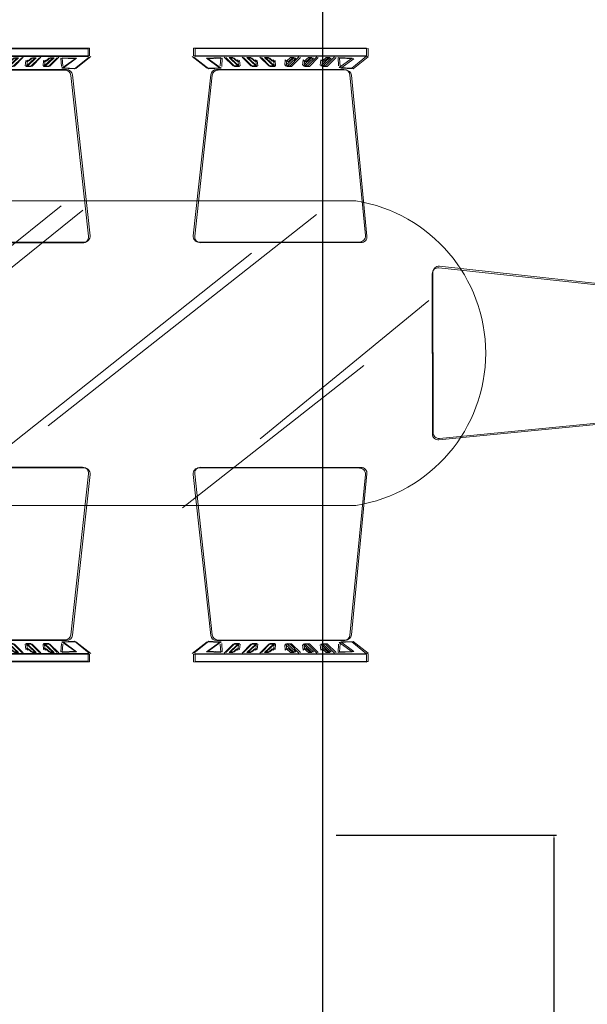
# Model space of a CAD drawing. Units: inches. Extents: x -26 to 575, y -18 to 513.
# Tile 20 of 28: x 316 to 355, y 241 to 307. Entities that reach past the tile are written whole.
import ezdxf

# ---------------------------------------------------------------- set-up
doc = ezdxf.new("R2010")
doc.units = ezdxf.units.IN
doc.header["$MEASUREMENT"] = 0
doc.layers.add('A-ANNO-DIMS', color=2, linetype='Continuous', lineweight=18)
doc.layers.add('Furniture', color=8, linetype='Continuous', lineweight=15)
doc.styles.get("Standard").update_dxf_attribs({"font": 'arial.ttf', "height": 6})
doc.dimstyles.get("Standard").update_dxf_attribs({"dimtxt": 6, "dimasz": 0.18, "dimexe": 0.18, "dimexo": 0.0625, "dimgap": 0.09, "dimtad": 0, "dimtih": 1, "dimtoh": 1, "dimzin": 0, "dimdsep": 46, "dimlunit": 3, "dimtxsty": 'Standard', "dimcen": 0.09, "dimadec": 0, "dimazin": 0, "dimtfac": 1, "dimtofl": 0, "dimtmove": 0, "dimatfit": 3, "dimfxl": 1, "dimtolj": 1, "dimtzin": 0, "dimarcsym": 0})

# ---------------------------------------------------------------- blocks, each defined once
blk = doc.blocks.new('DINING-SET-6-SEAT')
for p, q in [((16.828, 40.76, -3.573), (16.828, 41.278, -3.573)), ((16.828, 41.278, -3.573), (28.461, 41.278, -3.573)), ((16.931, 40.798, -3.573), (16.931, 41.316, -3.573)), ((16.931, 41.316, -3.573), (28.564, 41.316, -3.573)), ((28.461, 41.278, -3.573), (28.461, 40.76, -3.573)), ((28.564, 41.316, -3.573), (28.564, 40.798, -3.573)), ((47.187, 41.329, -3.573), (35.554, 41.319, -3.573)), ((35.554, 41.319, -3.573), (35.554, 40.801, -3.573)), ((47.29, 41.291, -3.573), (35.657, 41.281, -3.573)), ((35.657, 41.281, -3.573), (35.657, 40.763, -3.573)), ((47.188, 40.811, -3.573), (47.187, 41.329, -3.573)), ((47.29, 40.774, -3.573), (47.29, 41.291, -3.573)), ((28.461, 40.76, -3.573), (16.828, 40.76, -3.573)), ((16.828, 40.72, -3.573), (17.824, 39.924, -3.573)), ((28.564, 40.798, -3.573), (16.931, 40.798, -3.573)), ((16.931, 40.758, -3.573), (17.927, 39.962, -3.573)), ((17.784, 40.601, -3.573), (18.74, 40.641, -3.573)), ((18.661, 39.964, -3.573), (17.784, 40.601, -3.573)), ((17.887, 40.639, -3.573), (18.843, 40.679, -3.573)), ((18.763, 40.002, -3.573), (17.887, 40.639, -3.573)), ((18.74, 40.641, -3.573), (18.7, 40.083, -3.573)), ((18.843, 40.679, -3.573), (18.803, 40.121, -3.573)), ((18.979, 40.681, -3.573), (19.577, 40.083, -3.573)), ((19.082, 40.718, -3.573), (19.68, 40.121, -3.573)), ((19.896, 40.083, -3.573), (19.298, 40.641, -3.573)), ((19.298, 40.641, -3.573), (19.537, 40.641, -3.573)), ((19.998, 40.121, -3.573), (19.401, 40.679, -3.573)), ((19.401, 40.679, -3.573), (19.64, 40.679, -3.573)), ((19.537, 40.641, -3.573), (19.816, 40.402, -3.573)), ((19.64, 40.679, -3.573), (19.919, 40.44, -3.573)), ((19.816, 40.402, -3.573), (19.896, 40.481, -3.573)), ((19.896, 40.481, -3.573), (19.936, 40.123, -3.573)), ((19.919, 40.44, -3.573), (19.998, 40.519, -3.573)), ((19.998, 40.519, -3.573), (20.038, 40.161, -3.573)), ((20.175, 40.681, -3.573), (20.772, 40.083, -3.573)), ((20.277, 40.718, -3.573), (20.875, 40.121, -3.573)), ((21.091, 40.083, -3.573), (20.493, 40.641, -3.573)), ((20.493, 40.641, -3.573), (20.732, 40.641, -3.573)), ((21.194, 40.121, -3.573), (20.596, 40.679, -3.573)), ((20.596, 40.679, -3.573), (20.835, 40.679, -3.573)), ((20.732, 40.641, -3.573), (21.011, 40.402, -3.573)), ((20.835, 40.679, -3.573), (21.114, 40.44, -3.573)), ((21.011, 40.402, -3.573), (21.091, 40.481, -3.573)), ((21.091, 40.481, -3.573), (21.131, 40.123, -3.573)), ((21.114, 40.44, -3.573), (21.194, 40.519, -3.573)), ((21.194, 40.519, -3.573), (21.233, 40.161, -3.573)), ((21.37, 40.681, -3.573), (21.967, 40.083, -3.573)), ((21.473, 40.718, -3.573), (22.07, 40.121, -3.573)), ((22.286, 40.083, -3.573), (21.688, 40.641, -3.573)), ((21.688, 40.641, -3.573), (21.928, 40.641, -3.573)), ((22.389, 40.121, -3.573), (21.791, 40.679, -3.573)), ((21.791, 40.679, -3.573), (22.03, 40.679, -3.573)), ((21.928, 40.641, -3.573), (22.206, 40.402, -3.573)), ((22.03, 40.679, -3.573), (22.309, 40.44, -3.573)), ((22.206, 40.402, -3.573), (22.286, 40.481, -3.573)), ((22.286, 40.481, -3.573), (22.326, 40.123, -3.573)), ((22.309, 40.44, -3.573), (22.389, 40.519, -3.573)), ((22.389, 40.519, -3.573), (22.429, 40.161, -3.573)), ((23.083, 40.481, -3.573), (23.043, 40.123, -3.573)), ((23.083, 40.083, -3.573), (23.681, 40.641, -3.573)), ((23.163, 40.402, -3.573), (23.083, 40.481, -3.573)), ((23.186, 40.519, -3.573), (23.146, 40.161, -3.573)), ((23.441, 40.641, -3.573), (23.163, 40.402, -3.573)), ((23.186, 40.121, -3.573), (23.783, 40.679, -3.573)), ((23.265, 40.44, -3.573), (23.186, 40.519, -3.573)), ((23.544, 40.679, -3.573), (23.265, 40.44, -3.573)), ((23.999, 40.681, -3.573), (23.402, 40.083, -3.573)), ((23.681, 40.641, -3.573), (23.441, 40.641, -3.573)), ((24.102, 40.718, -3.573), (23.504, 40.121, -3.573)), ((23.783, 40.679, -3.573), (23.544, 40.679, -3.573)), ((24.278, 40.481, -3.573), (24.238, 40.123, -3.573)), ((24.278, 40.083, -3.573), (24.876, 40.641, -3.573)), ((24.358, 40.402, -3.573), (24.278, 40.481, -3.573)), ((24.381, 40.519, -3.573), (24.341, 40.161, -3.573)), ((24.637, 40.641, -3.573), (24.358, 40.402, -3.573)), ((24.381, 40.121, -3.573), (24.978, 40.679, -3.573)), ((24.461, 40.44, -3.573), (24.381, 40.519, -3.573)), ((24.739, 40.679, -3.573), (24.461, 40.44, -3.573)), ((25.194, 40.681, -3.573), (24.597, 40.083, -3.573)), ((24.876, 40.641, -3.573), (24.637, 40.641, -3.573)), ((25.297, 40.718, -3.573), (24.7, 40.121, -3.573)), ((24.978, 40.679, -3.573), (24.739, 40.679, -3.573)), ((25.473, 40.481, -3.573), (25.434, 40.123, -3.573)), ((25.473, 40.083, -3.573), (26.071, 40.641, -3.573)), ((25.553, 40.402, -3.573), (25.473, 40.481, -3.573)), ((25.576, 40.519, -3.573), (25.536, 40.161, -3.573)), ((25.832, 40.641, -3.573), (25.553, 40.402, -3.573)), ((25.576, 40.121, -3.573), (26.174, 40.679, -3.573)), ((25.656, 40.44, -3.573), (25.576, 40.519, -3.573)), ((25.935, 40.679, -3.573), (25.656, 40.44, -3.573)), ((26.39, 40.681, -3.573), (25.792, 40.083, -3.573)), ((26.071, 40.641, -3.573), (25.832, 40.641, -3.573)), ((26.492, 40.718, -3.573), (25.895, 40.121, -3.573)), ((26.174, 40.679, -3.573), (25.935, 40.679, -3.573)), ((27.585, 40.601, -3.573), (26.629, 40.641, -3.573)), ((26.629, 40.641, -3.573), (26.669, 40.083, -3.573)), ((26.708, 39.964, -3.573), (27.585, 40.601, -3.573)), ((27.688, 40.639, -3.573), (26.731, 40.679, -3.573)), ((26.731, 40.679, -3.573), (26.771, 40.121, -3.573)), ((26.811, 40.002, -3.573), (27.688, 40.639, -3.573)), ((28.541, 40.72, -3.573), (27.545, 39.924, -3.573)), ((28.644, 40.758, -3.573), (27.648, 39.962, -3.573)), ((35.475, 40.761, -3.573), (36.471, 39.966, -3.573)), ((35.554, 40.801, -3.573), (47.188, 40.811, -3.573)), ((35.577, 40.723, -3.573), (36.574, 39.928, -3.573)), ((35.657, 40.763, -3.573), (47.29, 40.774, -3.573)), ((36.431, 40.643, -3.573), (37.387, 40.683, -3.573)), ((37.308, 40.006, -3.573), (36.431, 40.643, -3.573)), ((36.534, 40.605, -3.573), (37.49, 40.646, -3.573)), ((37.411, 39.968, -3.573), (36.534, 40.605, -3.573)), ((37.387, 40.683, -3.573), (37.348, 40.126, -3.573)), ((37.49, 40.646, -3.573), (37.45, 40.088, -3.573)), ((37.626, 40.723, -3.573), (38.224, 40.127, -3.573)), ((37.729, 40.686, -3.573), (38.327, 40.089, -3.573)), ((38.543, 40.127, -3.573), (37.945, 40.684, -3.573)), ((37.945, 40.684, -3.573), (38.184, 40.684, -3.573)), ((38.646, 40.089, -3.573), (38.048, 40.646, -3.573)), ((38.048, 40.646, -3.573), (38.287, 40.646, -3.573)), ((38.184, 40.684, -3.573), (38.463, 40.445, -3.573)), ((38.287, 40.646, -3.573), (38.566, 40.408, -3.573)), ((38.463, 40.445, -3.573), (38.543, 40.525, -3.573)), ((38.543, 40.525, -3.573), (38.583, 40.167, -3.573)), ((38.566, 40.408, -3.573), (38.645, 40.487, -3.573)), ((38.645, 40.487, -3.573), (38.685, 40.129, -3.573)), ((38.821, 40.724, -3.573), (39.419, 40.128, -3.573)), ((38.924, 40.687, -3.573), (39.522, 40.09, -3.573)), ((39.738, 40.128, -3.573), (39.14, 40.685, -3.573)), ((39.14, 40.685, -3.573), (39.379, 40.685, -3.573)), ((39.841, 40.09, -3.573), (39.243, 40.647, -3.573)), ((39.243, 40.647, -3.573), (39.482, 40.647, -3.573)), ((39.379, 40.685, -3.573), (39.658, 40.446, -3.573)), ((39.482, 40.647, -3.573), (39.761, 40.409, -3.573)), ((39.658, 40.446, -3.573), (39.738, 40.526, -3.573)), ((39.738, 40.526, -3.573), (39.778, 40.168, -3.573)), ((39.761, 40.409, -3.573), (39.841, 40.488, -3.573)), ((39.841, 40.488, -3.573), (39.881, 40.13, -3.573)), ((40.016, 40.725, -3.573), (40.615, 40.129, -3.573)), ((40.119, 40.688, -3.573), (40.717, 40.091, -3.573)), ((40.933, 40.129, -3.573), (40.335, 40.686, -3.573)), ((40.335, 40.686, -3.573), (40.574, 40.686, -3.573)), ((41.036, 40.091, -3.573), (40.438, 40.648, -3.573)), ((40.438, 40.648, -3.573), (40.677, 40.648, -3.573)), ((40.574, 40.686, -3.573), (40.853, 40.447, -3.573)), ((40.677, 40.648, -3.573), (40.956, 40.41, -3.573)), ((40.853, 40.447, -3.573), (40.933, 40.527, -3.573)), ((40.933, 40.527, -3.573), (40.973, 40.169, -3.573)), ((40.956, 40.41, -3.573), (41.036, 40.489, -3.573)), ((41.036, 40.489, -3.573), (41.076, 40.131, -3.573)), ((41.73, 40.528, -3.573), (41.69, 40.169, -3.573)), ((41.73, 40.13, -3.573), (42.327, 40.688, -3.573)), ((41.81, 40.448, -3.573), (41.73, 40.528, -3.573)), ((41.833, 40.49, -3.573), (41.793, 40.132, -3.573)), ((42.088, 40.687, -3.573), (41.81, 40.448, -3.573)), ((41.833, 40.092, -3.573), (42.43, 40.65, -3.573)), ((41.912, 40.41, -3.573), (41.833, 40.49, -3.573)), ((42.191, 40.65, -3.573), (41.912, 40.41, -3.573)), ((42.646, 40.728, -3.573), (42.049, 40.13, -3.573)), ((42.327, 40.688, -3.573), (42.088, 40.687, -3.573)), ((42.749, 40.69, -3.573), (42.152, 40.092, -3.573)), ((42.43, 40.65, -3.573), (42.191, 40.65, -3.573)), ((42.925, 40.529, -3.573), (42.885, 40.17, -3.573)), ((42.925, 40.131, -3.573), (43.522, 40.689, -3.573)), ((43.005, 40.449, -3.573), (42.925, 40.529, -3.573)), ((43.028, 40.491, -3.573), (42.988, 40.133, -3.573)), ((43.283, 40.688, -3.573), (43.005, 40.449, -3.573)), ((43.028, 40.093, -3.573), (43.625, 40.651, -3.573)), ((43.108, 40.412, -3.573), (43.028, 40.491, -3.573)), ((43.386, 40.651, -3.573), (43.108, 40.412, -3.573)), ((43.841, 40.729, -3.573), (43.244, 40.131, -3.573)), ((43.522, 40.689, -3.573), (43.283, 40.688, -3.573)), ((43.944, 40.691, -3.573), (43.347, 40.093, -3.573)), ((43.625, 40.651, -3.573), (43.386, 40.651, -3.573)), ((44.12, 40.53, -3.573), (44.081, 40.171, -3.573)), ((44.2, 40.45, -3.573), (44.12, 40.53, -3.573)), ((44.121, 40.132, -3.573), (44.718, 40.69, -3.573)), ((44.223, 40.492, -3.573), (44.183, 40.134, -3.573)), ((44.479, 40.69, -3.573), (44.2, 40.45, -3.573)), ((44.223, 40.094, -3.573), (44.82, 40.652, -3.573)), ((44.303, 40.413, -3.573), (44.223, 40.492, -3.573)), ((44.581, 40.652, -3.573), (44.303, 40.413, -3.573)), ((45.036, 40.73, -3.573), (44.439, 40.132, -3.573)), ((44.718, 40.69, -3.573), (44.479, 40.69, -3.573)), ((45.139, 40.692, -3.573), (44.542, 40.094, -3.573)), ((44.82, 40.652, -3.573), (44.581, 40.652, -3.573)), ((46.232, 40.651, -3.573), (45.275, 40.69, -3.573)), ((45.275, 40.69, -3.573), (45.316, 40.133, -3.573)), ((45.356, 40.013, -3.573), (46.232, 40.651, -3.573)), ((46.334, 40.613, -3.573), (45.378, 40.652, -3.573)), ((45.378, 40.652, -3.573), (45.419, 40.095, -3.573)), ((45.458, 39.976, -3.573), (46.334, 40.613, -3.573)), ((47.188, 40.772, -3.573), (46.192, 39.974, -3.573)), ((47.29, 40.734, -3.573), (46.295, 39.936, -3.573)), ((17.824, 39.924, -3.573), (18.661, 39.964, -3.573)), ((17.927, 39.962, -3.573), (18.763, 40.002, -3.573)), ((26.909, 39.844, -3.573), (18.345, 39.844, -3.573)), ((27.012, 39.882, -3.573), (18.448, 39.882, -3.573)), ((19.577, 40.083, -3.573), (19.896, 40.083, -3.573)), ((19.68, 40.121, -3.573), (19.998, 40.121, -3.573)), ((20.772, 40.083, -3.573), (21.091, 40.083, -3.573)), ((20.875, 40.121, -3.573), (21.194, 40.121, -3.573)), ((21.967, 40.083, -3.573), (22.286, 40.083, -3.573)), ((22.07, 40.121, -3.573), (22.389, 40.121, -3.573)), ((23.402, 40.083, -3.573), (23.083, 40.083, -3.573)), ((23.504, 40.121, -3.573), (23.186, 40.121, -3.573)), ((24.597, 40.083, -3.573), (24.278, 40.083, -3.573)), ((24.7, 40.121, -3.573), (24.381, 40.121, -3.573)), ((25.792, 40.083, -3.573), (25.473, 40.083, -3.573)), ((25.895, 40.121, -3.573), (25.576, 40.121, -3.573)), ((27.545, 39.924, -3.573), (26.708, 39.964, -3.573)), ((27.648, 39.962, -3.573), (26.811, 40.002, -3.573)), ((36.471, 39.966, -3.573), (37.308, 40.006, -3.573)), ((36.574, 39.928, -3.573), (37.411, 39.968, -3.573)), ((37.107, 39.887, -3.573), (45.671, 39.894, -3.573)), ((37.21, 39.849, -3.573), (45.774, 39.856, -3.573)), ((38.224, 40.127, -3.573), (38.543, 40.127, -3.573)), ((38.327, 40.089, -3.573), (38.646, 40.089, -3.573)), ((39.419, 40.128, -3.573), (39.738, 40.128, -3.573)), ((39.522, 40.09, -3.573), (39.841, 40.09, -3.573)), ((40.615, 40.129, -3.573), (40.933, 40.129, -3.573)), ((40.717, 40.091, -3.573), (41.036, 40.091, -3.573)), ((42.049, 40.13, -3.573), (41.73, 40.13, -3.573)), ((42.152, 40.092, -3.573), (41.833, 40.092, -3.573)), ((43.244, 40.131, -3.573), (42.925, 40.131, -3.573)), ((43.347, 40.093, -3.573), (43.028, 40.093, -3.573)), ((44.439, 40.132, -3.573), (44.121, 40.132, -3.573)), ((44.542, 40.094, -3.573), (44.223, 40.094, -3.573)), ((46.192, 39.974, -3.573), (45.356, 40.013, -3.573)), ((46.295, 39.936, -3.573), (45.458, 39.976, -3.573)), ((17.949, 39.484, -3.573), (16.91, 28.653, -3.573)), ((18.052, 39.522, -3.573), (17.012, 28.691, -3.573)), ((28.493, 28.659, -3.573), (27.305, 39.489, -3.573)), ((28.595, 28.696, -3.573), (27.408, 39.527, -3.573)), ((35.534, 28.7, -3.573), (36.712, 39.531, -3.573)), ((35.636, 28.662, -3.573), (36.814, 39.494, -3.573)), ((46.068, 39.534, -3.573), (47.117, 28.704, -3.573)), ((46.171, 39.496, -3.573), (47.219, 28.667, -3.573)), ((16.194, 22.294, -1.308), (26.662, 30.717, -1.308)), ((46.474, 31.041, -1.308), (18.1, 31.041, -1.308)), ((14.74, 19.68, -1.308), (28.116, 30.426, -1.308)), ((25.79, 15.904, -1.308), (43.819, 30.136, -1.308)), ((17.306, 28.217, -3.573), (28.097, 28.217, -3.573)), ((17.409, 28.255, -3.573), (28.199, 28.255, -3.573)), ((46.72, 28.268, -3.573), (35.93, 28.258, -3.573)), ((46.823, 28.23, -3.573), (36.033, 28.22, -3.573)), ((18.1, 10.54, -1.308), (39.457, 27.522, -1.308)), ((0, 14.987, -3.573), (0.01, 26.621, -3.573)), ((0.01, 26.621, -3.573), (0.528, 26.62, -3.573)), ((0.037, 14.884, -3.573), (0.048, 26.518, -3.573)), ((0.048, 26.518, -3.573), (0.565, 26.517, -3.573)), ((0.528, 26.62, -3.573), (0.517, 14.987, -3.573)), ((0.565, 26.517, -3.573), (0.555, 14.884, -3.573)), ((0.567, 26.7, -3.573), (1.363, 25.703, -3.573)), ((0.605, 26.597, -3.573), (1.401, 25.6, -3.573)), ((12.629, 26.641, -3.573), (1.797, 25.463, -3.573)), ((12.667, 26.538, -3.573), (1.835, 25.36, -3.573)), ((52.057, 26.538, -3.573), (62.889, 25.36, -3.573)), ((52.095, 26.641, -3.573), (62.926, 25.463, -3.573)), ((64.119, 26.597, -3.573), (63.323, 25.6, -3.573)), ((64.156, 26.7, -3.573), (63.361, 25.703, -3.573)), ((64.676, 26.518, -3.573), (64.159, 26.517, -3.573)), ((64.159, 26.517, -3.573), (64.169, 14.884, -3.573)), ((64.714, 26.621, -3.573), (64.196, 26.62, -3.573)), ((64.196, 26.62, -3.573), (64.207, 14.987, -3.573)), ((64.686, 14.884, -3.573), (64.676, 26.518, -3.573)), ((64.724, 14.987, -3.573), (64.714, 26.621, -3.573)), ((13.061, 15.454, -3.573), (13.071, 26.244, -3.573)), ((13.099, 15.351, -3.573), (13.108, 26.142, -3.573)), ((51.625, 15.351, -3.573), (51.615, 26.142, -3.573)), ((51.663, 15.454, -3.573), (51.653, 26.244, -3.573)), ((0.686, 25.744, -3.573), (0.645, 24.787, -3.573)), ((0.724, 25.641, -3.573), (0.683, 24.685, -3.573)), ((1.322, 24.866, -3.573), (0.686, 25.744, -3.573)), ((1.36, 24.764, -3.573), (0.724, 25.641, -3.573)), ((1.363, 25.703, -3.573), (1.322, 24.866, -3.573)), ((1.401, 25.6, -3.573), (1.36, 24.764, -3.573)), ((63.323, 25.6, -3.573), (63.364, 24.764, -3.573)), ((63.361, 25.703, -3.573), (63.401, 24.866, -3.573)), ((63.364, 24.764, -3.573), (64, 25.641, -3.573)), ((63.401, 24.866, -3.573), (64.038, 25.744, -3.573)), ((64, 25.641, -3.573), (64.041, 24.685, -3.573)), ((64.038, 25.744, -3.573), (64.078, 24.787, -3.573)), ((0.605, 24.548, -3.573), (1.202, 23.95, -3.573)), ((0.645, 24.787, -3.573), (1.203, 24.827, -3.573)), ((0.683, 24.685, -3.573), (1.241, 24.724, -3.573)), ((1.442, 25.067, -3.573), (1.435, 16.503, -3.573)), ((1.48, 24.964, -3.573), (1.472, 16.401, -3.573)), ((63.244, 24.964, -3.573), (63.252, 16.401, -3.573)), ((63.282, 25.067, -3.573), (63.289, 16.503, -3.573)), ((64.041, 24.685, -3.573), (63.483, 24.724, -3.573)), ((64.078, 24.787, -3.573), (63.521, 24.827, -3.573)), ((64.118, 24.548, -3.573), (63.522, 23.95, -3.573)), ((0.643, 24.446, -3.573), (1.24, 23.847, -3.573)), ((1.202, 23.632, -3.573), (0.645, 24.23, -3.573)), ((0.645, 24.23, -3.573), (0.645, 23.991, -3.573)), ((0.645, 23.991, -3.573), (0.883, 23.712, -3.573)), ((0.683, 24.127, -3.573), (0.682, 23.888, -3.573)), ((0.682, 23.888, -3.573), (0.921, 23.609, -3.573)), ((1.24, 23.529, -3.573), (0.683, 24.127, -3.573)), ((1.202, 23.95, -3.573), (1.202, 23.632, -3.573)), ((40.039, 15.033, -1.308), (51.38, 24.327, -1.308)), ((64.081, 24.446, -3.573), (63.484, 23.847, -3.573)), ((63.484, 23.529, -3.573), (64.041, 24.127, -3.573)), ((63.522, 23.632, -3.573), (64.079, 24.23, -3.573)), ((63.522, 23.95, -3.573), (63.522, 23.632, -3.573)), ((64.041, 23.888, -3.573), (63.803, 23.609, -3.573)), ((64.079, 23.991, -3.573), (63.84, 23.712, -3.573)), ((64.041, 24.127, -3.573), (64.041, 23.888, -3.573)), ((64.079, 24.23, -3.573), (64.079, 23.991, -3.573)), ((0.604, 23.353, -3.573), (1.201, 22.755, -3.573)), ((0.642, 23.25, -3.573), (1.239, 22.652, -3.573)), ((0.883, 23.712, -3.573), (0.804, 23.632, -3.573)), ((0.804, 23.632, -3.573), (1.162, 23.592, -3.573)), ((0.921, 23.609, -3.573), (0.841, 23.529, -3.573)), ((0.841, 23.529, -3.573), (1.2, 23.489, -3.573)), ((1.24, 23.847, -3.573), (1.24, 23.529, -3.573)), ((63.484, 23.847, -3.573), (63.484, 23.529, -3.573)), ((64.082, 23.25, -3.573), (63.485, 22.652, -3.573)), ((64.12, 23.353, -3.573), (63.523, 22.755, -3.573)), ((63.882, 23.529, -3.573), (63.524, 23.489, -3.573)), ((63.92, 23.632, -3.573), (63.562, 23.592, -3.573)), ((63.803, 23.609, -3.573), (63.882, 23.529, -3.573)), ((63.84, 23.712, -3.573), (63.92, 23.632, -3.573)), ((1.201, 22.436, -3.573), (0.644, 23.034, -3.573)), ((0.644, 23.034, -3.573), (0.644, 22.795, -3.573)), ((0.644, 22.795, -3.573), (0.882, 22.516, -3.573)), ((0.682, 22.932, -3.573), (0.681, 22.693, -3.573)), ((0.681, 22.693, -3.573), (0.92, 22.414, -3.573)), ((1.239, 22.334, -3.573), (0.682, 22.932, -3.573)), ((1.201, 22.755, -3.573), (1.201, 22.436, -3.573)), ((1.239, 22.652, -3.573), (1.239, 22.334, -3.573)), ((63.485, 22.334, -3.573), (64.042, 22.932, -3.573)), ((63.485, 22.652, -3.573), (63.485, 22.334, -3.573)), ((63.523, 22.436, -3.573), (64.08, 23.034, -3.573)), ((63.523, 22.755, -3.573), (63.523, 22.436, -3.573)), ((64.042, 22.693, -3.573), (63.804, 22.414, -3.573)), ((64.08, 22.795, -3.573), (63.842, 22.516, -3.573)), ((64.042, 22.932, -3.573), (64.042, 22.693, -3.573)), ((64.08, 23.034, -3.573), (64.08, 22.795, -3.573)), ((0.603, 22.158, -3.573), (1.2, 21.56, -3.573)), ((0.641, 22.055, -3.573), (1.238, 21.457, -3.573)), ((0.882, 22.516, -3.573), (0.803, 22.437, -3.573)), ((0.803, 22.437, -3.573), (1.161, 22.397, -3.573)), ((0.92, 22.414, -3.573), (0.84, 22.334, -3.573)), ((0.84, 22.334, -3.573), (1.199, 22.294, -3.573)), ((64.083, 22.055, -3.573), (63.486, 21.457, -3.573)), ((64.121, 22.158, -3.573), (63.524, 21.56, -3.573)), ((63.883, 22.334, -3.573), (63.525, 22.294, -3.573)), ((63.921, 22.437, -3.573), (63.563, 22.397, -3.573)), ((63.804, 22.414, -3.573), (63.883, 22.334, -3.573)), ((63.842, 22.516, -3.573), (63.921, 22.437, -3.573)), ((1.2, 21.241, -3.573), (0.643, 21.839, -3.573)), ((0.643, 21.839, -3.573), (0.643, 21.6, -3.573)), ((0.643, 21.6, -3.573), (0.881, 21.321, -3.573)), ((0.681, 21.736, -3.573), (0.68, 21.497, -3.573)), ((0.68, 21.497, -3.573), (0.919, 21.218, -3.573)), ((1.238, 21.138, -3.573), (0.681, 21.736, -3.573)), ((0.881, 21.321, -3.573), (0.802, 21.241, -3.573)), ((0.802, 21.241, -3.573), (1.16, 21.201, -3.573)), ((0.919, 21.218, -3.573), (0.839, 21.139, -3.573)), ((1.2, 21.56, -3.573), (1.2, 21.241, -3.573)), ((1.238, 21.457, -3.573), (1.238, 21.138, -3.573)), ((63.486, 21.138, -3.573), (64.043, 21.736, -3.573)), ((63.486, 21.457, -3.573), (63.486, 21.138, -3.573)), ((63.524, 21.241, -3.573), (64.081, 21.839, -3.573)), ((63.524, 21.56, -3.573), (63.524, 21.241, -3.573)), ((63.922, 21.241, -3.573), (63.564, 21.201, -3.573)), ((64.043, 21.497, -3.573), (63.805, 21.218, -3.573)), ((63.805, 21.218, -3.573), (63.884, 21.139, -3.573)), ((64.081, 21.6, -3.573), (63.843, 21.321, -3.573)), ((63.843, 21.321, -3.573), (63.922, 21.241, -3.573)), ((64.043, 21.736, -3.573), (64.043, 21.497, -3.573)), ((64.081, 21.839, -3.573), (64.081, 21.6, -3.573)), ((0.839, 21.139, -3.573), (1.198, 21.099, -3.573)), ((63.884, 21.139, -3.573), (63.526, 21.099, -3.573)), ((0.601, 19.529, -3.573), (1.199, 20.126, -3.573)), ((0.639, 19.426, -3.573), (1.237, 20.023, -3.573)), ((1.199, 20.444, -3.573), (0.641, 19.847, -3.573)), ((0.641, 20.086, -3.573), (0.88, 20.365, -3.573)), ((0.641, 19.847, -3.573), (0.641, 20.086, -3.573)), ((1.237, 20.342, -3.573), (0.679, 19.744, -3.573)), ((0.679, 19.983, -3.573), (0.918, 20.262, -3.573)), ((0.679, 19.744, -3.573), (0.679, 19.983, -3.573)), ((0.801, 20.445, -3.573), (1.159, 20.484, -3.573)), ((0.88, 20.365, -3.573), (0.801, 20.445, -3.573)), ((0.839, 20.342, -3.573), (1.197, 20.381, -3.573)), ((0.918, 20.262, -3.573), (0.839, 20.342, -3.573)), ((1.199, 20.126, -3.573), (1.199, 20.444, -3.573)), ((1.237, 20.023, -3.573), (1.237, 20.342, -3.573)), ((34.805, 10.386, -1.308), (47.018, 19.971, -1.308)), ((63.487, 20.023, -3.573), (63.487, 20.342, -3.573)), ((63.487, 20.342, -3.573), (64.045, 19.744, -3.573)), ((64.085, 19.426, -3.573), (63.487, 20.023, -3.573)), ((63.525, 20.126, -3.573), (63.525, 20.444, -3.573)), ((63.525, 20.444, -3.573), (64.083, 19.847, -3.573)), ((64.123, 19.529, -3.573), (63.525, 20.126, -3.573)), ((63.885, 20.342, -3.573), (63.527, 20.381, -3.573)), ((63.923, 20.445, -3.573), (63.565, 20.484, -3.573)), ((63.806, 20.262, -3.573), (63.885, 20.342, -3.573)), ((64.045, 19.983, -3.573), (63.806, 20.262, -3.573)), ((63.843, 20.365, -3.573), (63.923, 20.445, -3.573)), ((64.083, 20.086, -3.573), (63.843, 20.365, -3.573)), ((64.045, 19.744, -3.573), (64.045, 19.983, -3.573)), ((64.083, 19.847, -3.573), (64.083, 20.086, -3.573)), ((1.198, 19.249, -3.573), (0.64, 18.652, -3.573)), ((0.8, 19.249, -3.573), (1.158, 19.289, -3.573)), ((0.879, 19.17, -3.573), (0.8, 19.249, -3.573)), ((1.198, 18.93, -3.573), (1.198, 19.249, -3.573)), ((63.526, 18.93, -3.573), (63.526, 19.249, -3.573)), ((63.526, 19.249, -3.573), (64.084, 18.652, -3.573)), ((63.924, 19.249, -3.573), (63.566, 19.289, -3.573)), ((63.844, 19.17, -3.573), (63.924, 19.249, -3.573)), ((0.6, 18.333, -3.573), (1.198, 18.93, -3.573)), ((0.638, 18.231, -3.573), (1.236, 18.828, -3.573)), ((0.64, 18.891, -3.573), (0.879, 19.17, -3.573)), ((0.64, 18.652, -3.573), (0.64, 18.891, -3.573)), ((1.236, 19.146, -3.573), (0.678, 18.549, -3.573)), ((0.678, 18.788, -3.573), (0.917, 19.067, -3.573)), ((0.678, 18.549, -3.573), (0.678, 18.788, -3.573)), ((0.838, 19.147, -3.573), (1.196, 19.186, -3.573)), ((0.917, 19.067, -3.573), (0.838, 19.147, -3.573)), ((1.236, 18.828, -3.573), (1.236, 19.146, -3.573)), ((63.488, 18.828, -3.573), (63.488, 19.146, -3.573)), ((63.488, 19.146, -3.573), (64.046, 18.549, -3.573)), ((64.086, 18.231, -3.573), (63.488, 18.828, -3.573)), ((64.124, 18.333, -3.573), (63.526, 18.93, -3.573)), ((63.886, 19.147, -3.573), (63.528, 19.186, -3.573)), ((63.807, 19.067, -3.573), (63.886, 19.147, -3.573)), ((64.046, 18.788, -3.573), (63.807, 19.067, -3.573)), ((64.084, 18.891, -3.573), (63.844, 19.17, -3.573)), ((64.046, 18.549, -3.573), (64.046, 18.788, -3.573)), ((64.084, 18.652, -3.573), (64.084, 18.891, -3.573)), ((1.197, 18.054, -3.573), (0.639, 17.457, -3.573)), ((0.639, 17.696, -3.573), (0.878, 17.974, -3.573)), ((1.235, 17.951, -3.573), (0.677, 17.354, -3.573)), ((0.799, 18.054, -3.573), (1.157, 18.094, -3.573)), ((0.878, 17.974, -3.573), (0.799, 18.054, -3.573)), ((0.837, 17.951, -3.573), (1.195, 17.991, -3.573)), ((0.916, 17.872, -3.573), (0.837, 17.951, -3.573)), ((1.197, 17.735, -3.573), (1.197, 18.054, -3.573)), ((1.234, 17.632, -3.573), (1.235, 17.951, -3.573)), ((63.489, 17.632, -3.573), (63.489, 17.951, -3.573)), ((63.489, 17.951, -3.573), (64.047, 17.354, -3.573)), ((63.527, 17.735, -3.573), (63.527, 18.054, -3.573)), ((63.527, 18.054, -3.573), (64.085, 17.457, -3.573)), ((63.887, 17.951, -3.573), (63.529, 17.991, -3.573)), ((63.925, 18.054, -3.573), (63.567, 18.094, -3.573)), ((63.808, 17.872, -3.573), (63.887, 17.951, -3.573)), ((63.846, 17.974, -3.573), (63.925, 18.054, -3.573)), ((64.085, 17.696, -3.573), (63.846, 17.974, -3.573)), ((0.599, 17.138, -3.573), (1.197, 17.735, -3.573)), ((0.637, 17.035, -3.573), (1.234, 17.632, -3.573)), ((0.639, 17.457, -3.573), (0.639, 17.696, -3.573)), ((0.677, 17.593, -3.573), (0.916, 17.872, -3.573)), ((0.677, 17.354, -3.573), (0.677, 17.593, -3.573)), ((64.087, 17.035, -3.573), (63.489, 17.632, -3.573)), ((64.125, 17.138, -3.573), (63.527, 17.735, -3.573)), ((64.047, 17.593, -3.573), (63.808, 17.872, -3.573)), ((64.047, 17.354, -3.573), (64.047, 17.593, -3.573)), ((64.085, 17.457, -3.573), (64.085, 17.696, -3.573)), ((0.677, 15.943, -3.573), (0.639, 16.899, -3.573)), ((0.639, 16.899, -3.573), (1.196, 16.859, -3.573)), ((0.715, 15.84, -3.573), (0.676, 16.796, -3.573)), ((0.676, 16.796, -3.573), (1.234, 16.756, -3.573)), ((1.315, 16.819, -3.573), (0.677, 15.943, -3.573)), ((1.353, 16.716, -3.573), (0.715, 15.84, -3.573)), ((1.354, 15.982, -3.573), (1.315, 16.819, -3.573)), ((1.392, 15.879, -3.573), (1.353, 16.716, -3.573)), ((63.332, 15.879, -3.573), (63.371, 16.716, -3.573)), ((63.369, 15.982, -3.573), (63.408, 16.819, -3.573)), ((63.371, 16.716, -3.573), (64.009, 15.84, -3.573)), ((63.408, 16.819, -3.573), (64.046, 15.943, -3.573)), ((64.048, 16.796, -3.573), (63.49, 16.756, -3.573)), ((64.085, 16.899, -3.573), (63.528, 16.859, -3.573)), ((64.009, 15.84, -3.573), (64.048, 16.796, -3.573)), ((64.046, 15.943, -3.573), (64.085, 16.899, -3.573)), ((0.557, 14.987, -3.573), (1.354, 15.982, -3.573)), ((1.795, 16.106, -3.573), (12.624, 15.058, -3.573)), ((1.832, 16.004, -3.573), (12.662, 14.955, -3.573)), ((62.892, 16.004, -3.573), (52.062, 14.955, -3.573)), ((62.929, 16.106, -3.573), (52.099, 15.058, -3.573)), ((64.167, 14.987, -3.573), (63.369, 15.982, -3.573)), ((0.595, 14.884, -3.573), (1.392, 15.879, -3.573)), ((64.129, 14.884, -3.573), (63.332, 15.879, -3.573)), ((0.517, 14.987, -3.573), (0, 14.987, -3.573)), ((0.555, 14.884, -3.573), (0.037, 14.884, -3.573)), ((64.169, 14.884, -3.573), (64.686, 14.884, -3.573)), ((64.207, 14.987, -3.573), (64.724, 14.987, -3.573)), ((17.949, 1.845, -3.573), (16.91, 12.676, -3.573)), ((18.052, 1.807, -3.573), (17.012, 12.638, -3.573)), ((17.306, 13.113, -3.573), (28.097, 13.113, -3.573)), ((17.409, 13.075, -3.573), (28.199, 13.075, -3.573)), ((28.493, 12.671, -3.573), (27.305, 1.84, -3.573)), ((28.595, 12.633, -3.573), (27.408, 1.802, -3.573)), ((35.534, 12.63, -3.573), (36.712, 1.798, -3.573)), ((35.636, 12.668, -3.573), (36.814, 1.836, -3.573)), ((46.72, 13.062, -3.573), (35.93, 13.071, -3.573)), ((46.823, 13.1, -3.573), (36.033, 13.109, -3.573)), ((46.068, 1.795, -3.573), (47.117, 12.625, -3.573)), ((46.171, 1.833, -3.573), (47.219, 12.663, -3.573)), ((18.1, 10.54, -1.308), (46.474, 10.54, -1.308)), ((16.828, 0.609, -3.573), (17.824, 1.405, -3.573)), ((16.931, 0.571, -3.573), (17.927, 1.367, -3.573)), ((18.661, 1.366, -3.573), (17.784, 0.728, -3.573)), ((17.824, 1.405, -3.573), (18.661, 1.366, -3.573)), ((18.763, 1.328, -3.573), (17.887, 0.691, -3.573)), ((17.927, 1.367, -3.573), (18.763, 1.328, -3.573)), ((26.909, 1.485, -3.573), (18.345, 1.485, -3.573)), ((27.012, 1.447, -3.573), (18.448, 1.447, -3.573)), ((27.545, 1.405, -3.573), (26.708, 1.366, -3.573)), ((26.708, 1.366, -3.573), (27.585, 0.728, -3.573)), ((27.648, 1.367, -3.573), (26.811, 1.328, -3.573)), ((26.811, 1.328, -3.573), (27.688, 0.691, -3.573)), ((28.541, 0.609, -3.573), (27.545, 1.405, -3.573)), ((28.644, 0.571, -3.573), (27.648, 1.367, -3.573)), ((35.475, 0.568, -3.573), (36.471, 1.364, -3.573)), ((35.577, 0.606, -3.573), (36.574, 1.401, -3.573)), ((36.471, 1.364, -3.573), (37.308, 1.323, -3.573)), ((37.411, 1.361, -3.573), (36.534, 0.724, -3.573)), ((36.574, 1.401, -3.573), (37.411, 1.361, -3.573)), ((37.107, 1.443, -3.573), (45.671, 1.435, -3.573)), ((37.21, 1.48, -3.573), (45.774, 1.473, -3.573)), ((46.192, 1.355, -3.573), (45.356, 1.316, -3.573)), ((46.295, 1.393, -3.573), (45.458, 1.354, -3.573)), ((45.458, 1.354, -3.573), (46.334, 0.716, -3.573)), ((47.188, 0.558, -3.573), (46.192, 1.355, -3.573)), ((47.29, 0.596, -3.573), (46.295, 1.393, -3.573)), ((17.784, 0.728, -3.573), (18.74, 0.689, -3.573)), ((17.887, 0.691, -3.573), (18.843, 0.651, -3.573)), ((18.74, 0.689, -3.573), (18.7, 1.246, -3.573)), ((18.843, 0.651, -3.573), (18.803, 1.208, -3.573)), ((18.979, 0.649, -3.573), (19.577, 1.246, -3.573)), ((19.082, 0.611, -3.573), (19.68, 1.208, -3.573)), ((19.896, 1.246, -3.573), (19.298, 0.689, -3.573)), ((19.298, 0.689, -3.573), (19.537, 0.689, -3.573)), ((19.998, 1.208, -3.573), (19.401, 0.651, -3.573)), ((19.537, 0.689, -3.573), (19.816, 0.928, -3.573)), ((19.577, 1.246, -3.573), (19.896, 1.246, -3.573)), ((19.64, 0.651, -3.573), (19.919, 0.89, -3.573)), ((19.68, 1.208, -3.573), (19.998, 1.208, -3.573)), ((19.816, 0.928, -3.573), (19.896, 0.848, -3.573)), ((19.896, 0.848, -3.573), (19.936, 1.206, -3.573)), ((19.919, 0.89, -3.573), (19.998, 0.81, -3.573)), ((19.998, 0.81, -3.573), (20.038, 1.168, -3.573)), ((20.175, 0.649, -3.573), (20.772, 1.246, -3.573)), ((20.277, 0.611, -3.573), (20.875, 1.208, -3.573)), ((21.091, 1.246, -3.573), (20.493, 0.689, -3.573)), ((20.493, 0.689, -3.573), (20.732, 0.689, -3.573)), ((21.194, 1.208, -3.573), (20.596, 0.651, -3.573)), ((20.732, 0.689, -3.573), (21.011, 0.928, -3.573)), ((20.772, 1.246, -3.573), (21.091, 1.246, -3.573)), ((20.835, 0.651, -3.573), (21.114, 0.89, -3.573)), ((20.875, 1.208, -3.573), (21.194, 1.208, -3.573)), ((21.011, 0.928, -3.573), (21.091, 0.848, -3.573)), ((21.091, 0.848, -3.573), (21.131, 1.206, -3.573)), ((21.114, 0.89, -3.573), (21.194, 0.81, -3.573)), ((21.194, 0.81, -3.573), (21.233, 1.168, -3.573)), ((21.37, 0.649, -3.573), (21.967, 1.246, -3.573)), ((21.473, 0.611, -3.573), (22.07, 1.208, -3.573)), ((22.286, 1.246, -3.573), (21.688, 0.689, -3.573)), ((21.688, 0.689, -3.573), (21.928, 0.689, -3.573)), ((22.389, 1.208, -3.573), (21.791, 0.651, -3.573)), ((21.928, 0.689, -3.573), (22.206, 0.928, -3.573)), ((21.967, 1.246, -3.573), (22.286, 1.246, -3.573)), ((22.03, 0.651, -3.573), (22.309, 0.89, -3.573)), ((22.07, 1.208, -3.573), (22.389, 1.208, -3.573)), ((22.206, 0.928, -3.573), (22.286, 0.848, -3.573)), ((22.286, 0.848, -3.573), (22.326, 1.206, -3.573)), ((22.309, 0.89, -3.573), (22.389, 0.81, -3.573)), ((22.389, 0.81, -3.573), (22.429, 1.168, -3.573)), ((23.083, 0.848, -3.573), (23.043, 1.206, -3.573)), ((23.402, 1.246, -3.573), (23.083, 1.246, -3.573)), ((23.083, 1.246, -3.573), (23.681, 0.689, -3.573)), ((23.163, 0.928, -3.573), (23.083, 0.848, -3.573)), ((23.186, 0.81, -3.573), (23.146, 1.168, -3.573)), ((23.441, 0.689, -3.573), (23.163, 0.928, -3.573)), ((23.504, 1.208, -3.573), (23.186, 1.208, -3.573)), ((23.186, 1.208, -3.573), (23.783, 0.651, -3.573)), ((23.265, 0.89, -3.573), (23.186, 0.81, -3.573)), ((23.544, 0.651, -3.573), (23.265, 0.89, -3.573)), ((23.999, 0.649, -3.573), (23.402, 1.246, -3.573)), ((23.681, 0.689, -3.573), (23.441, 0.689, -3.573)), ((24.102, 0.611, -3.573), (23.504, 1.208, -3.573)), ((24.278, 0.848, -3.573), (24.238, 1.206, -3.573)), ((24.597, 1.246, -3.573), (24.278, 1.246, -3.573)), ((24.278, 1.246, -3.573), (24.876, 0.689, -3.573)), ((24.358, 0.928, -3.573), (24.278, 0.848, -3.573)), ((24.381, 0.81, -3.573), (24.341, 1.168, -3.573)), ((24.637, 0.689, -3.573), (24.358, 0.928, -3.573)), ((24.7, 1.208, -3.573), (24.381, 1.208, -3.573)), ((24.381, 1.208, -3.573), (24.978, 0.651, -3.573)), ((24.461, 0.89, -3.573), (24.381, 0.81, -3.573)), ((24.739, 0.651, -3.573), (24.461, 0.89, -3.573)), ((25.194, 0.649, -3.573), (24.597, 1.246, -3.573)), ((24.876, 0.689, -3.573), (24.637, 0.689, -3.573)), ((25.297, 0.611, -3.573), (24.7, 1.208, -3.573)), ((25.473, 0.848, -3.573), (25.434, 1.206, -3.573)), ((25.792, 1.246, -3.573), (25.473, 1.246, -3.573)), ((25.473, 1.246, -3.573), (26.071, 0.689, -3.573)), ((25.553, 0.928, -3.573), (25.473, 0.848, -3.573)), ((25.576, 0.81, -3.573), (25.536, 1.168, -3.573)), ((25.832, 0.689, -3.573), (25.553, 0.928, -3.573)), ((25.895, 1.208, -3.573), (25.576, 1.208, -3.573)), ((25.576, 1.208, -3.573), (26.174, 0.651, -3.573)), ((25.656, 0.89, -3.573), (25.576, 0.81, -3.573)), ((25.935, 0.651, -3.573), (25.656, 0.89, -3.573)), ((26.39, 0.649, -3.573), (25.792, 1.246, -3.573)), ((26.071, 0.689, -3.573), (25.832, 0.689, -3.573)), ((26.492, 0.611, -3.573), (25.895, 1.208, -3.573)), ((26.629, 0.689, -3.573), (26.669, 1.246, -3.573)), ((27.585, 0.728, -3.573), (26.629, 0.689, -3.573)), ((26.731, 0.651, -3.573), (26.771, 1.208, -3.573)), ((27.688, 0.691, -3.573), (26.731, 0.651, -3.573)), ((37.308, 1.323, -3.573), (36.431, 0.687, -3.573)), ((36.431, 0.687, -3.573), (37.387, 0.646, -3.573)), ((36.534, 0.724, -3.573), (37.49, 0.684, -3.573)), ((37.387, 0.646, -3.573), (37.348, 1.204, -3.573)), ((37.49, 0.684, -3.573), (37.45, 1.241, -3.573)), ((37.626, 0.606, -3.573), (38.224, 1.203, -3.573)), ((37.729, 0.644, -3.573), (38.327, 1.241, -3.573)), ((38.543, 1.203, -3.573), (37.945, 0.646, -3.573)), ((38.646, 1.24, -3.573), (38.048, 0.683, -3.573)), ((38.048, 0.683, -3.573), (38.287, 0.683, -3.573)), ((38.184, 0.645, -3.573), (38.463, 0.884, -3.573)), ((38.224, 1.203, -3.573), (38.543, 1.203, -3.573)), ((38.287, 0.683, -3.573), (38.566, 0.922, -3.573)), ((38.327, 1.241, -3.573), (38.646, 1.24, -3.573)), ((38.463, 0.884, -3.573), (38.543, 0.804, -3.573)), ((38.543, 0.804, -3.573), (38.583, 1.163, -3.573)), ((38.566, 0.922, -3.573), (38.645, 0.842, -3.573)), ((38.645, 0.842, -3.573), (38.685, 1.2, -3.573)), ((38.821, 0.605, -3.573), (39.419, 1.202, -3.573)), ((38.924, 0.643, -3.573), (39.522, 1.24, -3.573)), ((39.738, 1.201, -3.573), (39.14, 0.645, -3.573)), ((39.841, 1.239, -3.573), (39.243, 0.682, -3.573)), ((39.243, 0.682, -3.573), (39.482, 0.682, -3.573)), ((39.379, 0.644, -3.573), (39.658, 0.883, -3.573)), ((39.419, 1.202, -3.573), (39.738, 1.201, -3.573)), ((39.482, 0.682, -3.573), (39.761, 0.921, -3.573)), ((39.522, 1.24, -3.573), (39.841, 1.239, -3.573)), ((39.658, 0.883, -3.573), (39.738, 0.803, -3.573)), ((39.738, 0.803, -3.573), (39.778, 1.162, -3.573)), ((39.761, 0.921, -3.573), (39.841, 0.841, -3.573)), ((39.841, 0.841, -3.573), (39.881, 1.199, -3.573)), ((40.016, 0.604, -3.573), (40.615, 1.201, -3.573)), ((40.119, 0.642, -3.573), (40.717, 1.238, -3.573)), ((40.933, 1.2, -3.573), (40.335, 0.643, -3.573)), ((41.036, 1.238, -3.573), (40.438, 0.681, -3.573)), ((40.438, 0.681, -3.573), (40.677, 0.681, -3.573)), ((40.574, 0.643, -3.573), (40.853, 0.882, -3.573)), ((40.615, 1.201, -3.573), (40.933, 1.2, -3.573)), ((40.677, 0.681, -3.573), (40.956, 0.92, -3.573)), ((40.717, 1.238, -3.573), (41.036, 1.238, -3.573)), ((40.853, 0.882, -3.573), (40.933, 0.802, -3.573)), ((40.933, 0.802, -3.573), (40.973, 1.161, -3.573)), ((40.956, 0.92, -3.573), (41.036, 0.84, -3.573)), ((41.036, 0.84, -3.573), (41.076, 1.198, -3.573)), ((41.73, 0.802, -3.573), (41.69, 1.16, -3.573)), ((42.049, 1.199, -3.573), (41.73, 1.2, -3.573)), ((41.73, 1.2, -3.573), (42.327, 0.642, -3.573)), ((41.81, 0.881, -3.573), (41.73, 0.802, -3.573)), ((41.833, 0.839, -3.573), (41.793, 1.198, -3.573)), ((42.088, 0.642, -3.573), (41.81, 0.881, -3.573)), ((42.152, 1.237, -3.573), (41.833, 1.238, -3.573)), ((41.833, 1.238, -3.573), (42.43, 0.679, -3.573)), ((41.912, 0.919, -3.573), (41.833, 0.839, -3.573)), ((42.191, 0.68, -3.573), (41.912, 0.919, -3.573)), ((42.646, 0.602, -3.573), (42.049, 1.199, -3.573)), ((42.749, 0.639, -3.573), (42.152, 1.237, -3.573)), ((42.43, 0.679, -3.573), (42.191, 0.68, -3.573)), ((42.925, 0.8, -3.573), (42.885, 1.159, -3.573)), ((43.244, 1.198, -3.573), (42.925, 1.199, -3.573)), ((42.925, 1.199, -3.573), (43.522, 0.641, -3.573)), ((43.005, 0.88, -3.573), (42.925, 0.8, -3.573)), ((43.028, 0.838, -3.573), (42.988, 1.197, -3.573)), ((43.283, 0.641, -3.573), (43.005, 0.88, -3.573)), ((43.347, 1.236, -3.573), (43.028, 1.236, -3.573)), ((43.028, 1.236, -3.573), (43.625, 0.678, -3.573)), ((43.108, 0.918, -3.573), (43.028, 0.838, -3.573)), ((43.386, 0.679, -3.573), (43.108, 0.918, -3.573)), ((43.841, 0.601, -3.573), (43.244, 1.198, -3.573)), ((43.944, 0.638, -3.573), (43.347, 1.236, -3.573)), ((43.625, 0.678, -3.573), (43.386, 0.679, -3.573)), ((44.12, 0.799, -3.573), (44.081, 1.158, -3.573)), ((44.2, 0.879, -3.573), (44.12, 0.799, -3.573)), ((44.439, 1.197, -3.573), (44.121, 1.198, -3.573)), ((44.121, 1.198, -3.573), (44.718, 0.64, -3.573)), ((44.223, 0.837, -3.573), (44.183, 1.196, -3.573)), ((44.479, 0.64, -3.573), (44.2, 0.879, -3.573)), ((44.542, 1.235, -3.573), (44.223, 1.235, -3.573)), ((44.223, 1.235, -3.573), (44.82, 0.677, -3.573)), ((44.303, 0.917, -3.573), (44.223, 0.837, -3.573)), ((44.581, 0.678, -3.573), (44.303, 0.917, -3.573)), ((45.036, 0.6, -3.573), (44.439, 1.197, -3.573)), ((45.139, 0.637, -3.573), (44.542, 1.235, -3.573)), ((44.82, 0.677, -3.573), (44.581, 0.678, -3.573)), ((45.275, 0.639, -3.573), (45.316, 1.197, -3.573)), ((46.232, 0.678, -3.573), (45.275, 0.639, -3.573)), ((45.356, 1.316, -3.573), (46.232, 0.678, -3.573)), ((45.378, 0.677, -3.573), (45.419, 1.234, -3.573)), ((46.334, 0.716, -3.573), (45.378, 0.677, -3.573)), ((28.461, 0.569, -3.573), (16.828, 0.569, -3.573)), ((16.828, 0.569, -3.573), (16.828, 0.051, -3.573)), ((16.828, 0.051, -3.573), (28.461, 0.051, -3.573)), ((28.564, 0.531, -3.573), (16.931, 0.531, -3.573)), ((16.931, 0.531, -3.573), (16.931, 0.014, -3.573)), ((16.931, 0.014, -3.573), (28.564, 0.014, -3.573)), ((19.401, 0.651, -3.573), (19.64, 0.651, -3.573)), ((20.596, 0.651, -3.573), (20.835, 0.651, -3.573)), ((21.791, 0.651, -3.573), (22.03, 0.651, -3.573)), ((23.783, 0.651, -3.573), (23.544, 0.651, -3.573)), ((24.978, 0.651, -3.573), (24.739, 0.651, -3.573)), ((26.174, 0.651, -3.573), (25.935, 0.651, -3.573)), ((28.461, 0.051, -3.573), (28.461, 0.569, -3.573)), ((28.564, 0.014, -3.573), (28.564, 0.531, -3.573)), ((35.554, 0.011, -3.573), (35.554, 0.528, -3.573)), ((35.554, 0.528, -3.573), (47.188, 0.518, -3.573)), ((47.187, 0, -3.573), (35.554, 0.011, -3.573)), ((35.657, 0.048, -3.573), (35.657, 0.566, -3.573)), ((35.657, 0.566, -3.573), (47.29, 0.556, -3.573)), ((47.29, 0.038, -3.573), (35.657, 0.048, -3.573)), ((37.945, 0.646, -3.573), (38.184, 0.645, -3.573)), ((39.14, 0.645, -3.573), (39.379, 0.644, -3.573)), ((40.335, 0.643, -3.573), (40.574, 0.643, -3.573)), ((42.327, 0.642, -3.573), (42.088, 0.642, -3.573)), ((43.522, 0.641, -3.573), (43.283, 0.641, -3.573)), ((44.718, 0.64, -3.573), (44.479, 0.64, -3.573)), ((47.188, 0.518, -3.573), (47.187, 0, -3.573)), ((47.29, 0.556, -3.573), (47.29, 0.038, -3.573))]:
    blk.add_line(p, q)
for centre, radius, start, end in [((18.345, 39.446, -3.573), 0.398, 90, 174.51988), ((18.448, 39.484, -3.573), 0.398, 90, 174.51988), ((26.909, 39.446, -3.573), 0.398, 6.25717, 90), ((27.012, 39.484, -3.573), 0.398, 6.25717, 90), ((37.108, 39.488, -3.573), 0.398, 90.05022, 173.79305), ((37.211, 39.45, -3.573), 0.398, 90.05022, 173.79305), ((45.671, 39.496, -3.573), 0.398, 5.53034, 90.05022), ((45.774, 39.458, -3.573), 0.398, 5.53034, 90.05022), ((19.748, 20.791, -1.308), 10.382, 99.13208, 260.86792), ((44.826, 20.791, -1.308), 10.382, 279.13208, 80.86792), ((17.306, 28.615, -3.573), 0.398, 174.51988, 270), ((17.409, 28.653, -3.573), 0.398, 174.51988, 270), ((28.097, 28.615, -3.573), 0.398, 270, 6.25717), ((28.199, 28.653, -3.573), 0.398, 270, 6.25717), ((35.93, 28.656, -3.573), 0.398, 173.79305, 270.05022), ((36.032, 28.619, -3.573), 0.398, 173.79305, 270.05022), ((46.72, 28.666, -3.573), 0.398, 270.05022, 5.53034), ((46.823, 28.628, -3.573), 0.398, 270.05022, 5.53034), ((12.672, 26.245, -3.573), 0.398, 359.94978, 96.20695), ((12.71, 26.142, -3.573), 0.398, 359.94978, 96.20695), ((52.014, 26.142, -3.573), 0.398, 83.79305, 180.05022), ((52.052, 26.245, -3.573), 0.398, 83.79305, 180.05022), ((1.84, 25.067, -3.573), 0.398, 96.20695, 179.94978), ((1.878, 24.964, -3.573), 0.398, 96.20695, 179.94978), ((62.846, 24.964, -3.573), 0.398, 0.05022, 83.79305), ((62.883, 25.067, -3.573), 0.398, 0.05022, 83.79305), ((1.833, 16.503, -3.573), 0.398, 179.94978, 264.46966), ((1.871, 16.4, -3.573), 0.398, 179.94978, 264.46966), ((62.853, 16.4, -3.573), 0.398, 275.53034, 0.05022), ((62.891, 16.503, -3.573), 0.398, 275.53034, 0.05022), ((12.663, 15.454, -3.573), 0.398, 264.46966, 359.94978), ((12.701, 15.352, -3.573), 0.398, 264.46966, 359.94978), ((52.023, 15.352, -3.573), 0.398, 180.05022, 275.53034), ((52.061, 15.454, -3.573), 0.398, 180.05022, 275.53034), ((17.306, 12.714, -3.573), 0.398, 90, 185.48012), ((17.409, 12.676, -3.573), 0.398, 90, 185.48012), ((28.097, 12.714, -3.573), 0.398, 353.74283, 90), ((28.199, 12.676, -3.573), 0.398, 353.74283, 90), ((35.93, 12.673, -3.573), 0.398, 89.94978, 186.20695), ((36.032, 12.711, -3.573), 0.398, 89.94978, 186.20695), ((46.72, 12.663, -3.573), 0.398, 354.46966, 89.94978), ((46.823, 12.701, -3.573), 0.398, 354.46966, 89.94978), ((18.345, 1.883, -3.573), 0.398, 185.48012, 270), ((18.448, 1.846, -3.573), 0.398, 185.48012, 270), ((26.909, 1.883, -3.573), 0.398, 270, 353.74283), ((27.012, 1.846, -3.573), 0.398, 270, 353.74283), ((37.108, 1.841, -3.573), 0.398, 186.20695, 269.94978), ((37.211, 1.879, -3.573), 0.398, 186.20695, 269.94978), ((45.671, 1.834, -3.573), 0.398, 269.94978, 354.46966), ((45.774, 1.871, -3.573), 0.398, 269.94978, 354.46966)]:
    blk.add_arc(centre, radius, start, end)
blk = doc.blocks.new('*D26')
at = {"layer": 'A-ANNO-DIMS', "color": 0, "lineweight": -2, "transparency": 16777216}
for p, q in [((337.628, 252.609), (352.461, 252.609)), ((352.281, 252.429), (352.281, 206.753)), ((352.281, 154.689), (352.281, 200.364)), ((337.628, 154.509), (352.461, 154.509))]:
    blk.add_line(p, q, dxfattribs=at)
at = {"layer": 'A-ANNO-DIMS', "color": 0, "transparency": 16777216}
for points in [[(352.251, 252.429), (352.311, 252.429), (352.281, 252.609)], [(352.251, 154.689), (352.311, 154.689), (352.281, 154.509)]]:
    blk.add_solid(points, dxfattribs=at)
at = {"layer": 'Defpoints', "color": 0, "transparency": 16777216}
for p in [(337.566, 252.609), (352.281, 252.609), (337.566, 154.509)]:
    blk.add_point(p, dxfattribs=at)
at = {"layer": 'A-ANNO-DIMS', "color": 0, "transparency": 16777216, "insert": (352.281, 203.559), "char_height": 6, "attachment_point": 5}
blk.add_mtext('\\A1;SECTIONAL SOFA 8\'-2" TYP.', dxfattribs=at)
blk = doc.blocks.new('*D31')
at = {"layer": 'A-ANNO-DIMS', "color": 0, "lineweight": -2, "transparency": 16777216}
for p, q in [((311.292, 466.445), (311.292, -8.972)), ((336.72, 466.445), (336.72, -8.972)), ((311.472, -8.792), (336.54, -8.792)), ((336.72, -8.792), (336.9, -8.792))]:
    blk.add_line(p, q, dxfattribs=at)
at = {"layer": 'A-ANNO-DIMS', "color": 0, "transparency": 16777216}
for points in [[(311.472, -8.762), (311.472, -8.822), (311.292, -8.792)], [(336.54, -8.762), (336.54, -8.822), (336.72, -8.792)]]:
    blk.add_solid(points, dxfattribs=at)
at = {"layer": 'Defpoints', "color": 0, "transparency": 16777216}
for p in [(311.292, 466.508), (336.72, 466.508), (336.72, -8.792)]:
    blk.add_point(p, dxfattribs=at)
at = {"layer": 'A-ANNO-DIMS', "color": 0, "transparency": 16777216, "insert": (352.006, -8.792), "char_height": 6, "attachment_point": 5}
blk.add_mtext('\\A1;2\'-1 1/2"', dxfattribs=at)

msp = doc.modelspace()

# ---------------------------------------------------------------- block references
at = {"layer": 'Furniture'}
msp.add_blockref('DINING-SET-6-SEAT', (292.485, 264.256), dxfattribs=at)

# ---------------------------------------------------------------- dimensions: what is measured, and where the dimension line sits
at = {"layer": 'A-ANNO-DIMS'}
dim = msp.add_linear_dim(base=(336.72, -8.792), p1=(311.292, 466.508), p2=(336.72, 466.508), dimstyle='Standard', override={"dimdec": 1, "dimlfac": 1, "dimrnd": 0, "dimzin": 1, "dimdsep": 46, "dimlunit": 4, "dimfrac": 2}, dxfattribs=at)
dim.commit()
dim.dimension.update_dxf_attribs({"geometry": '*D31', "text_midpoint": (352.006, -8.792)})
dim = msp.add_linear_dim(base=(352.281, 252.609), p1=(337.566, 154.509), p2=(337.566, 252.609), angle=90, text='SECTIONAL SOFA <> TYP.', dimstyle='Standard', override={"dimdec": 1, "dimlfac": 1, "dimrnd": 0, "dimzin": 1, "dimdsep": 46, "dimlunit": 4, "dimfrac": 2}, dxfattribs=at)
dim.commit()
dim.dimension.update_dxf_attribs({"geometry": '*D26', "text_midpoint": (352.281, 203.559)})

doc.saveas('drawing.dxf')
